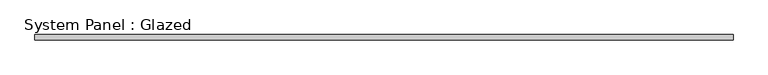
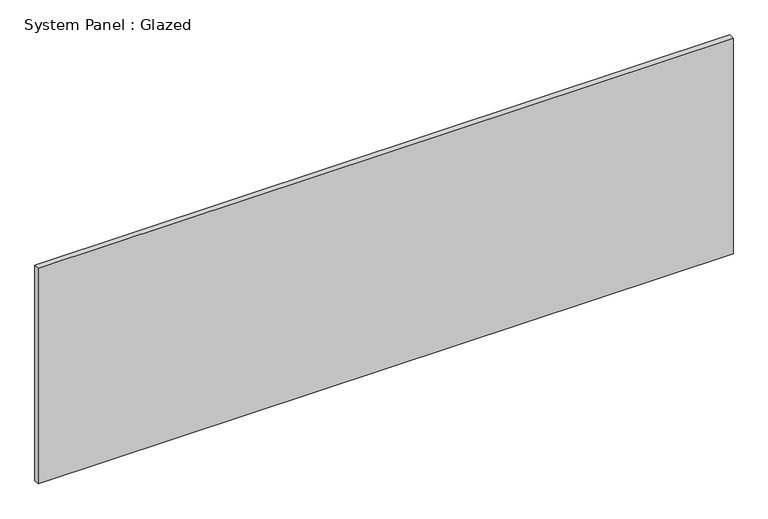
"""IFC4 building model written with IfcOpenShell, lengths in millimetres: plate geometry, System Panel : Glazed."""

from ifc_helpers import new_model, si_unit, origin, origin_with_axes, place, context, project, spatial, polyline, outline, extrude, source, transform, mapped, element, save


def system_panel_glazed_82fe4a0c(model_context):
    return source(origin(), model_context, "Body", "SweptSolid", [
        extrude(outline(polyline([(1606.55, 19.05), (-1606.55, 19.05), (-1606.55, 44.45), (1606.55, 44.45), (1606.55, 19.05)])), origin_with_axes(), (0.0, 0.0, 1.0), 1053.3367632),
    ])


if __name__ == "__main__":
    model = new_model("IFC4")
    model_context = context("Model", 3, world=origin())
    ifc_project = project(units=[si_unit("LENGTHUNIT", "METRE", prefix="MILLI")], contexts=[model_context])
    site = spatial("IfcSite", under=ifc_project)
    building = spatial("IfcBuilding", under=site)
    placement = place(None, origin())
    system_panel_glazed_shape = system_panel_glazed_82fe4a0c(model_context)
    element("IfcPlate", 1, ObjectType="System Panel : Glazed", at=placement, inside=building, context=model_context, shape_type="MappedRepresentation", body=[
        mapped(system_panel_glazed_shape, transform((0.0, 0.0, 0.0), x_axis=(1.0, 0.0, 0.0), y_axis=(0.0, 1.0, 0.0), z_axis=(0.0, 0.0, 1.0))),
    ])
    save(model, "model.ifc")

# Revit data of these elements
# Type "System Panel : Glazed"
#   Construction Type Id = "GSP4R"
#   Analytic Construction = "1/8 in Pilkington single glazing"
#   Visual Light Transmittance = 0.9
#   Solar Heat Gain Coefficient = 0.86
#   Heat Transfer Coefficient (U) = 1.18115 BTU/(h·ft²·°F)
#   Define Thermal Properties by = 1
# Element 1 (IfcPlate, "System Panel : Glazed")
#   Materials on its faces: "Glass"
# Materials
#   "Glass": class "Glass", colour RGB 0 128 192, transparency 0.75, Description = "Soda Lime Glass", Cost = 0
